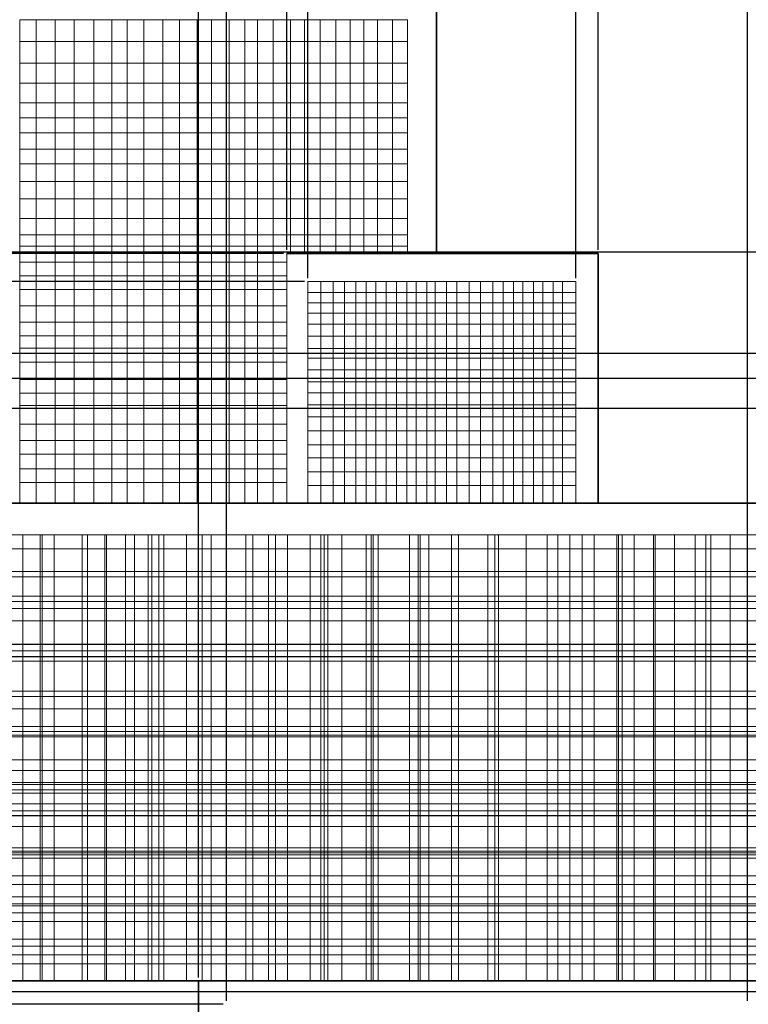
# Model space of a CAD drawing. Units: inches. Extents: x -10 to 130, y -32 to 34.
# Tile 9 of 22: x 28.66 to 42.14, y 5.57 to 23.78. Entities that reach past the tile are written whole.
import ezdxf

# ---------------------------------------------------------------- set-up
doc = ezdxf.new("R2010")
doc.units = ezdxf.units.IN
doc.header["$MEASUREMENT"] = 0
for name, color, linetype, lineweight in [('A-ANNO-DIMS', 2, 'Continuous', 18), ('A-ELEV', 7, 'Continuous', 35), ('A-GLAZ', 4, 'Continuous', 18)]:
    doc.layers.add(name, color=color, linetype=linetype, lineweight=lineweight)
doc.styles.get("Standard").update_dxf_attribs({"font": 'arial.ttf'})
doc.dimstyles.get("Standard").update_dxf_attribs({"dimtxt": 0.18, "dimasz": 0.18, "dimexe": 0.18, "dimexo": 0.0625, "dimgap": 0.09, "dimtad": 0, "dimtih": 1, "dimtoh": 1, "dimdec": 4, "dimzin": 0, "dimdsep": 46, "dimtxsty": 'Standard', "dimcen": 0.09, "dimadec": 0, "dimazin": 0, "dimtfac": 1, "dimtdec": 4, "dimtofl": 0, "dimtmove": 0, "dimatfit": 3, "dimfxl": 1, "dimtolj": 1, "dimtzin": 0, "dimarcsym": 0})

# ---------------------------------------------------------------- blocks, each defined once
blk = doc.blocks.new('*D5')
at = {"layer": 'A-ANNO-DIMS', "color": 0, "lineweight": -2, "transparency": 16777216}
for p, q in [((26.399, 6.07), (26.399, 33.879)), ((31.971, 6.07), (31.971, 33.879)), ((26.579, 33.699), (28.792, 33.699)), ((31.791, 33.699), (29.578, 33.699))]:
    blk.add_line(p, q, dxfattribs=at)
at = {"layer": 'A-ANNO-DIMS', "color": 0, "transparency": 16777216}
for points in [[(26.579, 33.729), (26.579, 33.669), (26.399, 33.699)], [(31.791, 33.729), (31.791, 33.669), (31.971, 33.699)]]:
    blk.add_solid(points, dxfattribs=at)
at = {"layer": 'Defpoints', "color": 0, "transparency": 16777216}
for p in [(31.971, 33.699), (26.399, 6.007), (31.971, 6.007)]:
    blk.add_point(p, dxfattribs=at)
at = {"layer": 'A-ANNO-DIMS', "color": 0, "transparency": 16777216, "insert": (29.185, 33.699), "char_height": 0.18, "attachment_point": 5}
blk.add_mtext('\\A1;5.572', dxfattribs=at)
blk = doc.blocks.new('*D6')
at = {"layer": 'A-ANNO-DIMS', "color": 0, "lineweight": -2, "transparency": 16777216}
for p, q in [((31.971, 6.07), (31.971, 33.879)), ((42.614, 6.07), (42.614, 33.879)), ((32.151, 33.699), (36.837, 33.699)), ((42.434, 33.699), (37.748, 33.699))]:
    blk.add_line(p, q, dxfattribs=at)
at = {"layer": 'A-ANNO-DIMS', "color": 0, "transparency": 16777216}
for points in [[(32.151, 33.729), (32.151, 33.669), (31.971, 33.699)], [(42.434, 33.729), (42.434, 33.669), (42.614, 33.699)]]:
    blk.add_solid(points, dxfattribs=at)
at = {"layer": 'Defpoints', "color": 0, "transparency": 16777216}
for p in [(42.614, 33.699), (31.971, 6.007), (42.614, 6.007)]:
    blk.add_point(p, dxfattribs=at)
at = {"layer": 'A-ANNO-DIMS', "color": 0, "transparency": 16777216, "insert": (37.293, 33.699), "char_height": 0.18, "attachment_point": 5}
blk.add_mtext('\\A1;10.643', dxfattribs=at)
blk = doc.blocks.new('*D14')
at = {"layer": 'A-ANNO-DIMS', "color": 0, "lineweight": -2, "transparency": 16777216}
for p, q in [((28.1, 24.464), (28.1, 33.879)), ((33.608, 19.52), (33.608, 33.879)), ((28.28, 33.699), (30.46, 33.699)), ((33.428, 33.699), (31.248, 33.699))]:
    blk.add_line(p, q, dxfattribs=at)
at = {"layer": 'A-ANNO-DIMS', "color": 0, "transparency": 16777216}
for points in [[(28.28, 33.729), (28.28, 33.669), (28.1, 33.699)], [(33.428, 33.729), (33.428, 33.669), (33.608, 33.699)]]:
    blk.add_solid(points, dxfattribs=at)
at = {"layer": 'Defpoints', "color": 0, "transparency": 16777216}
for p in [(33.608, 33.699), (28.1, 24.402), (33.608, 19.458)]:
    blk.add_point(p, dxfattribs=at)
at = {"layer": 'A-ANNO-DIMS', "color": 0, "transparency": 16777216, "insert": (30.854, 33.699), "char_height": 0.18, "attachment_point": 5}
blk.add_mtext('\\A1;5.508', dxfattribs=at)
blk = doc.blocks.new('*D15')
at = {"layer": 'A-ANNO-DIMS', "color": 0, "lineweight": -2, "transparency": 16777216}
for p, q in [((33.608, 19.52), (33.608, 33.879)), ((36.377, 24.464), (36.377, 33.879)), ((33.788, 33.699), (34.597, 33.699)), ((36.197, 33.699), (35.388, 33.699))]:
    blk.add_line(p, q, dxfattribs=at)
at = {"layer": 'A-ANNO-DIMS', "color": 0, "transparency": 16777216}
for points in [[(33.788, 33.729), (33.788, 33.669), (33.608, 33.699)], [(36.197, 33.729), (36.197, 33.669), (36.377, 33.699)]]:
    blk.add_solid(points, dxfattribs=at)
at = {"layer": 'Defpoints', "color": 0, "transparency": 16777216}
for p in [(36.377, 33.699), (36.377, 24.402), (33.608, 19.458)]:
    blk.add_point(p, dxfattribs=at)
at = {"layer": 'A-ANNO-DIMS', "color": 0, "transparency": 16777216, "insert": (34.993, 33.699), "char_height": 0.18, "attachment_point": 5}
blk.add_mtext('\\A1;2.769', dxfattribs=at)
blk = doc.blocks.new('*D16')
at = {"layer": 'A-ANNO-DIMS', "color": 0, "lineweight": -2, "transparency": 16777216}
for p, q in [((36.377, 24.464), (36.377, 33.879)), ((39.364, 19.52), (39.364, 33.879)), ((36.557, 33.699), (37.476, 33.699)), ((39.184, 33.699), (38.266, 33.699))]:
    blk.add_line(p, q, dxfattribs=at)
at = {"layer": 'A-ANNO-DIMS', "color": 0, "transparency": 16777216}
for points in [[(36.557, 33.729), (36.557, 33.669), (36.377, 33.699)], [(39.184, 33.729), (39.184, 33.669), (39.364, 33.699)]]:
    blk.add_solid(points, dxfattribs=at)
at = {"layer": 'Defpoints', "color": 0, "transparency": 16777216}
for p in [(39.364, 33.699), (36.377, 24.402), (39.364, 19.458)]:
    blk.add_point(p, dxfattribs=at)
at = {"layer": 'A-ANNO-DIMS', "color": 0, "transparency": 16777216, "insert": (37.871, 33.699), "char_height": 0.18, "attachment_point": 5}
blk.add_mtext('\\A1;2.987', dxfattribs=at)
blk = doc.blocks.new('*D17')
at = {"layer": 'A-ANNO-DIMS', "color": 0, "lineweight": -2, "transparency": 16777216}
for p, q in [((39.364, 19.52), (39.364, 33.879)), ((44.622, 17.67), (44.622, 33.879)), ((39.544, 33.699), (41.599, 33.699)), ((44.442, 33.699), (42.387, 33.699))]:
    blk.add_line(p, q, dxfattribs=at)
at = {"layer": 'A-ANNO-DIMS', "color": 0, "transparency": 16777216}
for points in [[(39.544, 33.729), (39.544, 33.669), (39.364, 33.699)], [(44.442, 33.729), (44.442, 33.669), (44.622, 33.699)]]:
    blk.add_solid(points, dxfattribs=at)
at = {"layer": 'Defpoints', "color": 0, "transparency": 16777216}
for p in [(44.622, 33.699), (39.364, 19.458), (44.622, 17.607)]:
    blk.add_point(p, dxfattribs=at)
at = {"layer": 'A-ANNO-DIMS', "color": 0, "transparency": 16777216, "insert": (41.993, 33.699), "char_height": 0.18, "attachment_point": 5}
blk.add_mtext('\\A1;5.257', dxfattribs=at)
blk = doc.blocks.new('*D28')
at = {"layer": 'A-ANNO-DIMS', "color": 0, "lineweight": -2, "transparency": 16777216}
for p, q in [((21.715, 14.903), (21.715, 33.879)), ((49.946, 14.903), (49.946, 33.879)), ((21.895, 33.699), (35.436, 33.699)), ((49.766, 33.699), (36.226, 33.699))]:
    blk.add_line(p, q, dxfattribs=at)
at = {"layer": 'A-ANNO-DIMS', "color": 0, "transparency": 16777216}
for points in [[(21.895, 33.729), (21.895, 33.669), (21.715, 33.699)], [(49.766, 33.729), (49.766, 33.669), (49.946, 33.699)]]:
    blk.add_solid(points, dxfattribs=at)
at = {"layer": 'Defpoints', "color": 0, "transparency": 16777216}
for p in [(49.946, 33.699), (21.715, 14.841), (49.946, 14.841)]:
    blk.add_point(p, dxfattribs=at)
at = {"layer": 'A-ANNO-DIMS', "color": 0, "transparency": 16777216, "insert": (35.831, 33.699), "char_height": 0.18, "attachment_point": 5}
blk.add_mtext('\\A1;28.23', dxfattribs=at)
blk = doc.blocks.new('*D34')
at = {"layer": 'A-ANNO-DIMS', "color": 0, "lineweight": -2, "transparency": 16777216}
for p, q in [((13.34, 6.007), (-9.564, 6.007)), ((-9.384, 5.827), (-9.384, 3.941)), ((-9.384, 1.691), (-9.384, 3.577)), ((70.835, 1.511), (-9.564, 1.511))]:
    blk.add_line(p, q, dxfattribs=at)
at = {"layer": 'A-ANNO-DIMS', "color": 0, "transparency": 16777216}
for points in [[(-9.414, 5.827), (-9.354, 5.827), (-9.384, 6.007)], [(-9.414, 1.691), (-9.354, 1.691), (-9.384, 1.511)]]:
    blk.add_solid(points, dxfattribs=at)
at = {"layer": 'Defpoints', "color": 0, "transparency": 16777216}
for p in [(-9.384, 6.007), (13.402, 6.007), (70.898, 1.511)]:
    blk.add_point(p, dxfattribs=at)
at = {"layer": 'A-ANNO-DIMS', "color": 0, "transparency": 16777216, "insert": (-9.384, 3.759), "char_height": 0.18, "attachment_point": 5}
blk.add_mtext('\\A1;4.497', dxfattribs=at)
blk = doc.blocks.new('*D36')
at = {"layer": 'A-ANNO-DIMS', "color": 0, "lineweight": -2, "transparency": 16777216}
for p, q in [((44.559, 17.607), (-9.564, 17.607)), ((-9.384, 17.427), (-9.384, 16.405)), ((-9.384, 15.021), (-9.384, 16.044)), ((21.653, 14.841), (-9.564, 14.841))]:
    blk.add_line(p, q, dxfattribs=at)
at = {"layer": 'A-ANNO-DIMS', "color": 0, "transparency": 16777216}
for points in [[(-9.414, 17.427), (-9.354, 17.427), (-9.384, 17.607)], [(-9.414, 15.021), (-9.354, 15.021), (-9.384, 14.841)]]:
    blk.add_solid(points, dxfattribs=at)
at = {"layer": 'Defpoints', "color": 0, "transparency": 16777216}
for p in [(-9.384, 17.607), (44.622, 17.607), (21.715, 14.841)]:
    blk.add_point(p, dxfattribs=at)
at = {"layer": 'A-ANNO-DIMS', "color": 0, "transparency": 16777216, "insert": (-9.384, 16.224), "char_height": 0.18, "attachment_point": 5}
blk.add_mtext('\\A1;2.77', dxfattribs=at)
blk = doc.blocks.new('*D37')
at = {"layer": 'A-ANNO-DIMS', "color": 0, "lineweight": -2, "transparency": 16777216}
for p, q in [((19.526, 19.485), (-9.564, 19.485)), ((-9.384, 19.305), (-9.384, 18.728)), ((-9.384, 17.787), (-9.384, 18.364)), ((44.559, 17.607), (-9.564, 17.607))]:
    blk.add_line(p, q, dxfattribs=at)
at = {"layer": 'A-ANNO-DIMS', "color": 0, "transparency": 16777216}
for points in [[(-9.414, 19.305), (-9.354, 19.305), (-9.384, 19.485)], [(-9.414, 17.787), (-9.354, 17.787), (-9.384, 17.607)]]:
    blk.add_solid(points, dxfattribs=at)
at = {"layer": 'Defpoints', "color": 0, "transparency": 16777216}
for p in [(-9.384, 19.485), (19.588, 19.485), (44.622, 17.607)]:
    blk.add_point(p, dxfattribs=at)
at = {"layer": 'A-ANNO-DIMS', "color": 0, "transparency": 16777216, "insert": (-9.384, 18.546), "char_height": 0.18, "attachment_point": 5}
blk.add_mtext('\\A1;1.877', dxfattribs=at)
blk = doc.blocks.new('*D74')
at = {"layer": 'A-ANNO-DIMS', "color": 0, "lineweight": -2, "transparency": 16777216}
for p, q in [((54.085, 17.607), (-9.564, 17.607)), ((-9.384, 17.427), (-9.384, 17.281)), ((-9.384, 16.771), (-9.384, 16.917)), ((55.856, 16.591), (-9.564, 16.591))]:
    blk.add_line(p, q, dxfattribs=at)
at = {"layer": 'A-ANNO-DIMS', "color": 0, "transparency": 16777216}
for points in [[(-9.414, 17.427), (-9.354, 17.427), (-9.384, 17.607)], [(-9.414, 16.771), (-9.354, 16.771), (-9.384, 16.591)]]:
    blk.add_solid(points, dxfattribs=at)
at = {"layer": 'Defpoints', "color": 0, "transparency": 16777216}
for p in [(54.147, 17.607), (-9.384, 16.591), (55.918, 16.591)]:
    blk.add_point(p, dxfattribs=at)
at = {"layer": 'A-ANNO-DIMS', "color": 0, "transparency": 16777216, "insert": (-9.384, 17.099), "char_height": 0.18, "attachment_point": 5}
blk.add_mtext('\\A1;1.02', dxfattribs=at)
blk = doc.blocks.new('*D82')
at = {"layer": 'A-ANNO-DIMS', "color": 0, "lineweight": -2, "transparency": 16777216}
for p, q in [((19.651, 19.485), (129.508, 19.485)), ((129.328, 19.305), (129.328, 18.728)), ((129.328, 17.787), (129.328, 18.364)), ((68.738, 17.607), (129.508, 17.607))]:
    blk.add_line(p, q, dxfattribs=at)
at = {"layer": 'A-ANNO-DIMS', "color": 0, "transparency": 16777216}
for points in [[(129.298, 19.305), (129.358, 19.305), (129.328, 19.485)], [(129.298, 17.787), (129.358, 17.787), (129.328, 17.607)]]:
    blk.add_solid(points, dxfattribs=at)
at = {"layer": 'Defpoints', "color": 0, "transparency": 16777216}
for p in [(19.588, 19.485), (68.676, 17.607), (129.328, 17.607)]:
    blk.add_point(p, dxfattribs=at)
at = {"layer": 'A-ANNO-DIMS', "color": 0, "transparency": 16777216, "insert": (129.328, 18.546), "char_height": 0.18, "attachment_point": 5}
blk.add_mtext('\\A1;1.877', dxfattribs=at)
blk = doc.blocks.new('*D87')
at = {"layer": 'A-ANNO-DIMS', "color": 0, "lineweight": -2, "transparency": 16777216}
for p, q in [((49.884, 14.841), (-9.564, 14.841)), ((-9.384, 14.661), (-9.384, 13.713)), ((-9.384, 12.402), (-9.384, 13.35)), ((49.884, 12.222), (-9.564, 12.222))]:
    blk.add_line(p, q, dxfattribs=at)
at = {"layer": 'A-ANNO-DIMS', "color": 0, "transparency": 16777216}
for points in [[(-9.414, 14.661), (-9.354, 14.661), (-9.384, 14.841)], [(-9.414, 12.402), (-9.354, 12.402), (-9.384, 12.222)]]:
    blk.add_solid(points, dxfattribs=at)
at = {"layer": 'Defpoints', "color": 0, "transparency": 16777216}
for p in [(49.946, 14.841), (-9.384, 12.222), (49.946, 12.222)]:
    blk.add_point(p, dxfattribs=at)
at = {"layer": 'A-ANNO-DIMS', "color": 0, "transparency": 16777216, "insert": (-9.384, 13.532), "char_height": 0.18, "attachment_point": 5}
blk.add_mtext('\\A1;2.619', dxfattribs=at)
blk = doc.blocks.new('*D88')
at = {"layer": 'A-ANNO-DIMS', "color": 0, "lineweight": -2, "transparency": 16777216}
for p, q in [((49.884, 12.222), (-9.564, 12.222)), ((-9.384, 12.042), (-9.384, 10.822)), ((-9.384, 9.238), (-9.384, 10.458)), ((49.884, 9.058), (-9.564, 9.058))]:
    blk.add_line(p, q, dxfattribs=at)
at = {"layer": 'A-ANNO-DIMS', "color": 0, "transparency": 16777216}
for points in [[(-9.414, 12.042), (-9.354, 12.042), (-9.384, 12.222)], [(-9.414, 9.238), (-9.354, 9.238), (-9.384, 9.058)]]:
    blk.add_solid(points, dxfattribs=at)
at = {"layer": 'Defpoints', "color": 0, "transparency": 16777216}
for p in [(49.946, 12.222), (-9.384, 9.058), (49.946, 9.058)]:
    blk.add_point(p, dxfattribs=at)
at = {"layer": 'A-ANNO-DIMS', "color": 0, "transparency": 16777216, "insert": (-9.384, 10.64), "char_height": 0.18, "attachment_point": 5}
blk.add_mtext('\\A1;3.164', dxfattribs=at)
blk = doc.blocks.new('*D89')
at = {"layer": 'A-ANNO-DIMS', "color": 0, "lineweight": -2, "transparency": 16777216}
for p, q in [((49.884, 9.058), (-9.564, 9.058)), ((-9.384, 8.878), (-9.384, 7.612)), ((-9.384, 5.982), (-9.384, 7.248)), ((49.884, 5.802), (-9.564, 5.802))]:
    blk.add_line(p, q, dxfattribs=at)
at = {"layer": 'A-ANNO-DIMS', "color": 0, "transparency": 16777216}
for points in [[(-9.414, 8.878), (-9.354, 8.878), (-9.384, 9.058)], [(-9.414, 5.982), (-9.354, 5.982), (-9.384, 5.802)]]:
    blk.add_solid(points, dxfattribs=at)
at = {"layer": 'Defpoints', "color": 0, "transparency": 16777216}
for p in [(49.946, 9.058), (-9.384, 5.802), (49.946, 5.802)]:
    blk.add_point(p, dxfattribs=at)
at = {"layer": 'A-ANNO-DIMS', "color": 0, "transparency": 16777216, "insert": (-9.384, 7.43), "char_height": 0.18, "attachment_point": 5}
blk.add_mtext('\\A1;3.256', dxfattribs=at)
blk = doc.blocks.new('*D90')
at = {"layer": 'A-ANNO-DIMS', "color": 0, "lineweight": -2, "transparency": 16777216}
for p, q in [((49.884, 5.802), (-9.564, 5.802)), ((-9.384, 5.622), (-9.384, 4.421)), ((-9.384, 2.855), (-9.384, 4.057)), ((49.884, 2.675), (-9.564, 2.675))]:
    blk.add_line(p, q, dxfattribs=at)
at = {"layer": 'A-ANNO-DIMS', "color": 0, "transparency": 16777216}
for points in [[(-9.414, 5.622), (-9.354, 5.622), (-9.384, 5.802)], [(-9.414, 2.855), (-9.354, 2.855), (-9.384, 2.675)]]:
    blk.add_solid(points, dxfattribs=at)
at = {"layer": 'Defpoints', "color": 0, "transparency": 16777216}
for p in [(49.946, 5.802), (-9.384, 2.675), (49.946, 2.675)]:
    blk.add_point(p, dxfattribs=at)
at = {"layer": 'A-ANNO-DIMS', "color": 0, "transparency": 16777216, "insert": (-9.384, 4.239), "char_height": 0.18, "attachment_point": 5}
blk.add_mtext('\\A1;3.127', dxfattribs=at)
blk = doc.blocks.new('*D95')
at = {"layer": 'A-ANNO-DIMS', "color": 0, "lineweight": -2, "transparency": 16777216}
for p, q in [((-9.384, 12.402), (-9.384, 12.582)), ((49.884, 12.222), (-9.564, 12.222)), ((49.884, 11.995), (-9.564, 11.995)), ((-9.384, 11.815), (-9.384, 11.635)), ((-9.384, 11.635), (-9.564, 11.635))]:
    blk.add_line(p, q, dxfattribs=at)
at = {"layer": 'A-ANNO-DIMS', "color": 0, "transparency": 16777216}
for points in [[(-9.414, 12.402), (-9.354, 12.402), (-9.384, 12.222)], [(-9.414, 11.815), (-9.354, 11.815), (-9.384, 11.995)]]:
    blk.add_solid(points, dxfattribs=at)
at = {"layer": 'Defpoints', "color": 0, "transparency": 16777216}
for p in [(49.946, 12.222), (-9.384, 11.995), (49.946, 11.995)]:
    blk.add_point(p, dxfattribs=at)
at = {"layer": 'A-ANNO-DIMS', "color": 0, "transparency": 16777216, "insert": (-9.957, 11.635), "char_height": 0.18, "attachment_point": 5}
blk.add_mtext('\\A1;0.227', dxfattribs=at)
blk = doc.blocks.new('*D102')
at = {"layer": 'A-ANNO-DIMS', "color": 0, "lineweight": -2, "transparency": 16777216}
for p, q in [((33.608, 19.52), (33.608, 33.879)), ((33.994, 18.998), (33.994, 33.879)), ((33.428, 33.699), (33.248, 33.699)), ((34.174, 33.699), (34.354, 33.699))]:
    blk.add_line(p, q, dxfattribs=at)
at = {"layer": 'A-ANNO-DIMS', "color": 0, "transparency": 16777216}
for points in [[(33.428, 33.729), (33.428, 33.669), (33.608, 33.699)], [(34.174, 33.729), (34.174, 33.669), (33.994, 33.699)]]:
    blk.add_solid(points, dxfattribs=at)
at = {"layer": 'Defpoints', "color": 0, "transparency": 16777216}
for p in [(33.994, 33.699), (33.608, 19.458), (33.994, 18.936)]:
    blk.add_point(p, dxfattribs=at)
at = {"layer": 'A-ANNO-DIMS', "color": 0, "transparency": 16777216, "insert": (34.748, 33.699), "char_height": 0.18, "attachment_point": 5}
blk.add_mtext('\\A1;0.386', dxfattribs=at)
blk = doc.blocks.new('*D103')
at = {"layer": 'A-ANNO-DIMS', "color": 0, "lineweight": -2, "transparency": 16777216}
for p, q in [((33.994, 18.998), (33.994, 33.879)), ((38.954, 18.998), (38.954, 33.879)), ((34.174, 33.699), (36.077, 33.699)), ((38.774, 33.699), (36.871, 33.699))]:
    blk.add_line(p, q, dxfattribs=at)
at = {"layer": 'A-ANNO-DIMS', "color": 0, "transparency": 16777216}
for points in [[(34.174, 33.729), (34.174, 33.669), (33.994, 33.699)], [(38.774, 33.729), (38.774, 33.669), (38.954, 33.699)]]:
    blk.add_solid(points, dxfattribs=at)
at = {"layer": 'Defpoints', "color": 0, "transparency": 16777216}
for p in [(38.954, 33.699), (33.994, 18.936), (38.954, 18.936)]:
    blk.add_point(p, dxfattribs=at)
at = {"layer": 'A-ANNO-DIMS', "color": 0, "transparency": 16777216, "insert": (36.474, 33.699), "char_height": 0.18, "attachment_point": 5}
blk.add_mtext('\\A1;4.960', dxfattribs=at)
blk = doc.blocks.new('*D104')
at = {"layer": 'A-ANNO-DIMS', "color": 0, "lineweight": -2, "transparency": 16777216}
for p, q in [((-9.383551, 19.637521), (-9.383551, 19.817521)), ((33.54566, 19.457521), (-9.563551, 19.457521)), ((33.931459, 18.935883), (-9.563551, 18.935883)), ((-9.383551, 18.755883), (-9.383551, 18.575883))]:
    blk.add_line(p, q, dxfattribs=at)
at = {"layer": 'A-ANNO-DIMS', "color": 0, "transparency": 16777216}
for points in [[(-9.413551, 19.637521), (-9.353551, 19.637521), (-9.383551, 19.457521)], [(-9.413551, 18.755883), (-9.353551, 18.755883), (-9.383551, 18.935883)]]:
    blk.add_solid(points, dxfattribs=at)
at = {"layer": 'Defpoints', "color": 0, "transparency": 16777216}
for p in [(-9.383551, 19.457521), (33.60816, 19.457521), (33.993959, 18.935883)]:
    blk.add_point(p, dxfattribs=at)
at = {"layer": 'A-ANNO-DIMS', "color": 0, "transparency": 16777216, "insert": (-9.383551, 19.196702), "char_height": 0.18, "attachment_point": 5}
blk.add_mtext('\\A1;0.522', dxfattribs=at)
blk = doc.blocks.new('*D106')
at = {"layer": 'A-ANNO-DIMS', "color": 0, "lineweight": -2, "transparency": 16777216}
for p, q in [((22.665, 14.318), (22.665, 33.879)), ((48.963, 14.318), (48.963, 33.879)), ((22.845, 33.699), (35.349, 33.699)), ((48.783, 33.699), (36.279, 33.699))]:
    blk.add_line(p, q, dxfattribs=at)
at = {"layer": 'A-ANNO-DIMS', "color": 0, "transparency": 16777216}
for points in [[(22.845, 33.729), (22.845, 33.669), (22.665, 33.699)], [(48.783, 33.729), (48.783, 33.669), (48.963, 33.699)]]:
    blk.add_solid(points, dxfattribs=at)
at = {"layer": 'Defpoints', "color": 0, "transparency": 16777216}
for p in [(48.963, 33.699), (22.665, 14.256), (48.963, 14.256)]:
    blk.add_point(p, dxfattribs=at)
at = {"layer": 'A-ANNO-DIMS', "color": 0, "transparency": 16777216, "insert": (35.814, 33.699), "char_height": 0.18, "attachment_point": 5}
blk.add_mtext('\\A1;26.298', dxfattribs=at)
blk = doc.blocks.new('*D110')
at = {"layer": 'A-ANNO-DIMS', "color": 0, "lineweight": -2, "transparency": 16777216}
for p, q in [((-9.383551, 17.787359), (-9.383551, 17.967359)), ((44.559228, 17.607359), (-9.563551, 17.607359)), ((45.040057, 17.142679), (-9.563551, 17.142679)), ((-9.383551, 16.962679), (-9.383551, 16.782679))]:
    blk.add_line(p, q, dxfattribs=at)
at = {"layer": 'A-ANNO-DIMS', "color": 0, "transparency": 16777216}
for points in [[(-9.413551, 17.787359), (-9.353551, 17.787359), (-9.383551, 17.607359)], [(-9.413551, 16.962679), (-9.353551, 16.962679), (-9.383551, 17.142679)]]:
    blk.add_solid(points, dxfattribs=at)
at = {"layer": 'Defpoints', "color": 0, "transparency": 16777216}
for p in [(-9.383551, 17.607359), (44.621728, 17.607359), (45.102557, 17.142679)]:
    blk.add_point(p, dxfattribs=at)
at = {"layer": 'A-ANNO-DIMS', "color": 0, "transparency": 16777216, "insert": (-9.383551, 17.375019), "char_height": 0.18, "attachment_point": 5}
blk.add_mtext('\\A1;0.465', dxfattribs=at)
blk = doc.blocks.new('*D119')
at = {"layer": 'A-ANNO-DIMS', "color": 0, "lineweight": -2, "transparency": 16777216}
for p, q in [((31.971, 6.07), (31.971, 33.879)), ((32.49, 5.634), (32.49, 33.879)), ((31.791, 33.699), (31.611, 33.699)), ((32.67, 33.699), (32.85, 33.699))]:
    blk.add_line(p, q, dxfattribs=at)
at = {"layer": 'A-ANNO-DIMS', "color": 0, "transparency": 16777216}
for points in [[(31.791, 33.729), (31.791, 33.669), (31.971, 33.699)], [(32.67, 33.729), (32.67, 33.669), (32.49, 33.699)]]:
    blk.add_solid(points, dxfattribs=at)
at = {"layer": 'Defpoints', "color": 0, "transparency": 16777216}
for p in [(32.49, 33.699), (31.971, 6.007), (32.49, 5.572)]:
    blk.add_point(p, dxfattribs=at)
at = {"layer": 'A-ANNO-DIMS', "color": 0, "transparency": 16777216, "insert": (33.244, 33.699), "char_height": 0.18, "attachment_point": 5}
blk.add_mtext('\\A1;0.519', dxfattribs=at)
blk = doc.blocks.new('*D120')
at = {"layer": 'A-ANNO-DIMS', "color": 0, "lineweight": -2, "transparency": 16777216}
for p, q in [((32.49, 5.634), (32.49, 33.879)), ((42.127, 5.634), (42.127, 33.879)), ((32.67, 33.699), (36.915, 33.699)), ((41.947, 33.699), (37.702, 33.699))]:
    blk.add_line(p, q, dxfattribs=at)
at = {"layer": 'A-ANNO-DIMS', "color": 0, "transparency": 16777216}
for points in [[(32.67, 33.729), (32.67, 33.669), (32.49, 33.699)], [(41.947, 33.729), (41.947, 33.669), (42.127, 33.699)]]:
    blk.add_solid(points, dxfattribs=at)
at = {"layer": 'Defpoints', "color": 0, "transparency": 16777216}
for p in [(42.127, 33.699), (32.49, 5.572), (42.127, 5.572)]:
    blk.add_point(p, dxfattribs=at)
at = {"layer": 'A-ANNO-DIMS', "color": 0, "transparency": 16777216, "insert": (37.308, 33.699), "char_height": 0.18, "attachment_point": 5}
blk.add_mtext('\\A1;9.637', dxfattribs=at)
blk = doc.blocks.new('*D121')
at = {"layer": 'A-ANNO-DIMS', "color": 0, "lineweight": -2, "transparency": 16777216}
for p, q in [((-9.384, 6.187), (-9.384, 6.367)), ((31.909, 6.007), (-9.564, 6.007)), ((32.427, 5.572), (-9.564, 5.572)), ((-9.384, 5.392), (-9.384, 5.212))]:
    blk.add_line(p, q, dxfattribs=at)
at = {"layer": 'A-ANNO-DIMS', "color": 0, "transparency": 16777216}
for points in [[(-9.414, 6.187), (-9.354, 6.187), (-9.384, 6.007)], [(-9.414, 5.392), (-9.354, 5.392), (-9.384, 5.572)]]:
    blk.add_solid(points, dxfattribs=at)
at = {"layer": 'Defpoints', "color": 0, "transparency": 16777216}
for p in [(-9.384, 6.007), (31.971, 6.007), (32.49, 5.572)]:
    blk.add_point(p, dxfattribs=at)
at = {"layer": 'A-ANNO-DIMS', "color": 0, "transparency": 16777216, "insert": (-9.384, 5.789), "char_height": 0.18, "attachment_point": 5}
blk.add_mtext('\\A1;0.436', dxfattribs=at)

msp = doc.modelspace()

# ---------------------------------------------------------------- linework, layer by layer
at = {"layer": 'A-ELEV'}
for p, q in [((36.3774, 24.4019), (36.3774, 19.4575)), ((36.3774, 19.4575), (33.6082, 19.4575)), ((36.3774, 19.4575), (39.3644, 19.4575)), ((39.3644, 19.4575), (39.3644, 14.8409)), ((21.7155, 14.8409), (49.9462, 14.8409)), ((20.3124, 6.0074), (49.9462, 6.0074)), ((31.9712, -6.2218), (31.9712, 6.0074))]:
    msp.add_line(p, q, dxfattribs=at)
at = {"layer": 'A-GLAZ'}
for p, q in [((28.6645, 23.7785), (28.6645, 14.8409)), ((28.6645, 23.7785), (35.841, 23.7785)), ((28.9723, 23.7785), (28.9723, 14.8409)), ((29.321, 23.7785), (29.321, 14.8409)), ((29.6697, 23.7785), (29.6697, 14.8409)), ((30.039, 23.7785), (30.039, 14.8409)), ((30.3672, 23.7785), (30.3672, 14.8409)), ((30.6545, 23.7785), (30.6545, 14.8409)), ((30.9622, 23.7785), (30.9622, 14.8409)), ((31.3109, 23.7785), (31.3109, 14.8409)), ((31.6186, 23.7785), (31.6186, 14.8409)), ((31.9469, 23.7785), (31.9469, 14.8409)), ((32.2136, 23.7785), (32.2136, 14.8409)), ((32.5418, 23.7785), (32.5418, 14.8409)), ((32.829, 23.7785), (32.829, 14.8409)), ((33.0672, 23.7785), (33.0672, 14.8409)), ((33.3515, 23.7785), (33.3515, 14.8409)), ((33.6779, 23.7785), (33.6779, 19.4575)), ((33.9309, 23.7785), (33.9309, 19.4575)), ((34.2218, 23.7785), (34.2218, 19.4575)), ((34.5128, 23.7785), (34.5128, 19.4575)), ((34.7784, 23.7785), (34.7784, 19.4575)), ((35.0314, 23.7785), (35.0314, 19.4575)), ((35.2844, 23.7785), (35.2844, 19.4575)), ((35.5627, 23.7785), (35.5627, 19.4575)), ((35.841, 23.7785), (35.841, 19.4575)), ((28.6645, 23.3752), (35.841, 23.3752)), ((28.6645, 22.9718), (35.841, 22.9718)), ((28.6645, 22.6051), (35.841, 22.6051)), ((28.6645, 22.2381), (35.841, 22.2381)), ((28.6645, 21.9622), (35.841, 21.9622)), ((28.6645, 21.6862), (35.841, 21.6862)), ((28.6645, 21.3872), (35.841, 21.3872)), ((28.6645, 21.1112), (35.841, 21.1112)), ((28.6645, 20.7893), (35.841, 20.7893)), ((28.6645, 20.4673), (35.841, 20.4673)), ((28.6645, 20.0993), (35.841, 20.0993)), ((28.6645, 19.8003), (35.841, 19.8003)), ((28.6645, 19.5933), (35.841, 19.5933)), ((33.6082, 19.4575), (33.6082, 14.8409)), ((28.6645, 19.2944), (33.6082, 19.2944)), ((28.6645, 19.0414), (33.6082, 19.0414)), ((36.3774, 18.9359), (33.994, 18.9359)), ((33.994, 18.9359), (33.994, 14.8409)), ((34.2385, 18.9359), (34.2385, 14.8409)), ((34.4656, 18.9359), (34.4656, 14.8409)), ((34.6752, 18.9359), (34.6752, 14.8409)), ((34.8848, 18.9359), (34.8848, 14.8409)), ((35.0769, 18.9359), (35.0769, 14.8409)), ((35.2515, 18.9359), (35.2515, 14.8409)), ((35.4437, 18.9359), (35.4437, 14.8409)), ((35.6358, 18.9359), (35.6358, 14.8409)), ((35.8279, 18.9359), (35.8279, 14.8409)), ((36.0026, 18.9359), (36.0026, 14.8409)), ((36.1947, 18.9359), (36.1947, 14.8409)), ((36.3519, 18.9359), (36.3519, 14.8409)), ((36.3774, 18.9359), (38.9544, 18.9359)), ((36.5615, 18.9359), (36.5615, 14.8409)), ((36.7537, 18.9359), (36.7537, 14.8409)), ((36.9807, 18.9359), (36.9807, 14.8409)), ((37.1903, 18.9359), (37.1903, 14.8409)), ((37.4171, 18.9359), (37.4171, 14.8409)), ((37.6092, 18.9359), (37.6092, 14.8409)), ((37.8013, 18.9359), (37.8013, 14.8409)), ((37.976, 18.9359), (37.976, 14.8409)), ((38.1681, 18.9359), (38.1681, 14.8409)), ((38.3428, 18.9359), (38.3428, 14.8409)), ((38.5349, 18.9359), (38.5349, 14.8409)), ((38.7096, 18.9359), (38.7096, 14.8409)), ((38.9544, 18.9359), (38.9544, 14.8409)), ((28.6645, 18.7884), (33.6082, 18.7884)), ((36.3774, 18.7336), (33.994, 18.7336)), ((36.3774, 18.7336), (38.9544, 18.7336)), ((28.6645, 18.4894), (33.6082, 18.4894)), ((36.3774, 18.5419), (33.994, 18.5419)), ((36.3774, 18.5419), (38.9544, 18.5419)), ((36.3774, 18.3502), (33.994, 18.3502)), ((36.3774, 18.3502), (38.9544, 18.3502)), ((28.6645, 18.1847), (33.6082, 18.1847)), ((36.3774, 18.1479), (33.994, 18.1479)), ((36.3774, 18.1479), (38.9544, 18.1479)), ((28.6645, 17.9317), (33.6082, 17.9317)), ((36.3774, 17.9243), (33.994, 17.9243)), ((36.3774, 17.9243), (38.9544, 17.9243)), ((28.6645, 17.7017), (33.6082, 17.7017)), ((36.3774, 17.7007), (33.994, 17.7007)), ((36.3774, 17.7007), (38.9544, 17.7007)), ((36.3774, 17.5197), (33.994, 17.5197)), ((36.3774, 17.5197), (38.9544, 17.5197)), ((28.6645, 17.4487), (33.6082, 17.4487)), ((36.3774, 17.3067), (33.994, 17.3067)), ((36.3774, 17.3067), (38.9544, 17.3067)), ((28.6645, 17.1267), (33.6082, 17.1267)), ((36.3774, 17.0831), (33.994, 17.0831)), ((36.3774, 17.0831), (38.9544, 17.0831)), ((28.6645, 16.8738), (33.6082, 16.8738)), ((36.3774, 16.8808), (33.994, 16.8808)), ((36.3774, 16.8808), (38.9544, 16.8808)), ((28.6645, 16.6438), (33.6082, 16.6438)), ((36.3774, 16.6571), (33.994, 16.6571)), ((36.3774, 16.6571), (38.9544, 16.6571)), ((36.3774, 16.4335), (33.994, 16.4335)), ((36.3774, 16.4335), (38.9544, 16.4335)), ((28.6645, 16.2988), (33.6082, 16.2988)), ((36.3774, 16.1747), (33.994, 16.1747)), ((36.3774, 16.1747), (38.9544, 16.1747)), ((28.6645, 15.9998), (33.6082, 15.9998)), ((36.3774, 15.9192), (33.994, 15.9192)), ((36.3774, 15.9192), (38.9544, 15.9192)), ((28.6645, 15.7469), (33.6082, 15.7469)), ((36.3774, 15.6742), (33.994, 15.6742)), ((36.3774, 15.6742), (38.9544, 15.6742)), ((28.6645, 15.4709), (33.6082, 15.4709)), ((36.3774, 15.4187), (33.994, 15.4187)), ((36.3774, 15.4187), (38.9544, 15.4187)), ((28.6645, 15.2179), (33.6082, 15.2179)), ((36.3774, 15.1631), (33.994, 15.1631)), ((36.3774, 15.1631), (38.9544, 15.1631)), ((22.6649, 14.2556), (48.963, 14.2556)), ((28.7237, 6.0074), (28.7237, 14.2556)), ((28.7237, 6.0074), (28.7237, 14.2556)), ((29.046, 6.0074), (29.046, 14.2556)), ((29.0782, 6.0074), (29.0782, 14.2556)), ((29.3038, 6.0074), (29.3038, 14.2556)), ((29.8195, 6.0074), (29.8195, 14.2556)), ((29.9162, 6.0074), (29.9162, 14.2556)), ((30.2385, 6.0074), (30.2385, 14.2556)), ((30.2707, 6.0074), (30.2707, 14.2556)), ((30.6252, 6.0074), (30.6252, 14.2556)), ((30.7863, 6.0074), (30.7863, 14.2556)), ((30.7863, 6.0074), (30.7863, 14.2556)), ((31.0442, 6.0074), (31.0442, 14.2556)), ((31.1086, 6.0074), (31.1086, 14.2556)), ((31.2375, 6.0074), (31.2375, 14.2556)), ((31.3342, 6.0074), (31.3342, 14.2556)), ((31.7532, 6.0074), (31.7532, 14.2556)), ((32.0432, 6.0074), (32.0432, 14.2556)), ((32.2044, 6.0074), (32.2044, 14.2556)), ((32.8489, 6.0074), (32.8489, 14.2556)), ((32.9778, 6.0074), (32.9778, 14.2556)), ((33.2679, 6.0074), (33.2679, 14.2556)), ((33.2679, 6.0074), (33.2679, 14.2556)), ((33.3968, 6.0074), (33.3968, 14.2556)), ((33.6224, 6.0074), (33.6224, 14.2556)), ((34.0414, 6.0074), (34.0414, 14.2556)), ((34.2347, 6.0074), (34.2347, 14.2556)), ((34.2992, 6.0074), (34.2992, 14.2556)), ((34.3637, 6.0074), (34.3637, 14.2556)), ((34.6215, 6.0074), (34.6215, 14.2556)), ((35.0727, 6.0074), (35.0727, 14.2556)), ((35.1694, 6.0074), (35.1694, 14.2556)), ((35.2016, 6.0074), (35.2016, 14.2556)), ((35.2983, 6.0074), (35.2983, 14.2556)), ((35.8784, 6.0074), (35.8784, 14.2556)), ((36.0395, 6.0074), (36.0395, 14.2556)), ((36.0717, 6.0074), (36.0717, 14.2556)), ((36.2329, 6.0074), (36.2329, 14.2556)), ((36.6519, 6.0074), (36.6519, 14.2556)), ((36.6519, 6.0074), (36.6519, 14.2556)), ((36.7808, 6.0074), (36.7808, 14.2556)), ((37.3286, 6.0074), (37.3286, 14.2556)), ((37.3286, 6.0074), (37.3286, 14.2556)), ((37.4576, 6.0074), (37.4576, 14.2556)), ((37.522, 6.0074), (37.522, 14.2556)), ((38.0377, 6.0074), (38.0377, 14.2556)), ((38.4244, 6.0074), (38.4244, 14.2556)), ((38.4244, 6.0074), (38.4244, 14.2556)), ((38.6178, 6.0074), (38.6178, 14.2556)), ((38.8434, 6.0074), (38.8434, 14.2556)), ((39.069, 6.0074), (39.069, 14.2556)), ((39.2946, 6.0074), (39.2946, 14.2556)), ((39.7135, 6.0074), (39.7135, 14.2556)), ((39.7457, 6.0074), (39.7457, 14.2556)), ((39.8102, 6.0074), (39.8102, 14.2556)), ((40.0358, 6.0074), (40.0358, 14.2556)), ((40.3903, 6.0074), (40.3903, 14.2556)), ((40.4225, 6.0074), (40.4225, 14.2556)), ((40.777, 6.0074), (40.777, 14.2556)), ((41.1638, 6.0074), (41.1638, 14.2556)), ((41.3572, 6.0074), (41.3572, 14.2556)), ((41.4538, 6.0074), (41.4538, 14.2556)), ((41.8083, 6.0074), (41.8083, 14.2556)), ((22.6649, 13.9954), (48.963, 13.9954)), ((22.6649, 13.5727), (48.963, 13.5727)), ((22.6649, 13.4751), (48.963, 13.4751)), ((22.6649, 13.1174), (48.963, 13.1174)), ((22.6649, 13.0199), (48.963, 13.0199)), ((22.6649, 12.8898), (48.963, 12.8898)), ((22.6649, 12.8898), (48.963, 12.8898)), ((22.6649, 12.6622), (48.963, 12.6622)), ((22.6649, 12.1093), (48.963, 12.1093)), ((22.6649, 11.9142), (48.963, 11.9142)), ((22.6649, 11.3614), (48.963, 11.3614)), ((22.6649, 11.3614), (48.963, 11.3614)), ((22.6649, 11.2638), (48.963, 11.2638)), ((22.6649, 11.0362), (48.963, 11.0362)), ((22.6649, 10.711), (48.963, 10.711)), ((22.6649, 10.711), (48.963, 10.711)), ((22.6649, 10.711), (48.963, 10.711)), ((22.6649, 10.6134), (48.963, 10.6134)), ((22.6649, 10.5484), (48.963, 10.5484)), ((22.6649, 10.5159), (48.963, 10.5159)), ((22.6649, 10.0931), (48.963, 10.0931)), ((22.6649, 9.898), (48.963, 9.898)), ((22.6649, 9.6704), (48.963, 9.6704)), ((22.6649, 9.6379), (48.963, 9.6379)), ((22.6649, 9.5403), (48.963, 9.5403)), ((22.6649, 9.4753), (48.963, 9.4753)), ((22.6649, 9.2802), (48.963, 9.2802)), ((22.6649, 9.1501), (48.963, 9.1501)), ((22.6649, 8.8574), (48.963, 8.8574)), ((22.6649, 8.4672), (48.963, 8.4672)), ((22.6649, 8.4021), (48.963, 8.4021)), ((22.6649, 8.3696), (48.963, 8.3696)), ((22.6649, 8.3371), (48.963, 8.3371)), ((22.6649, 8.2721), (48.963, 8.2721)), ((22.6649, 7.9469), (48.963, 7.9469)), ((22.6649, 7.7843), (48.963, 7.7843)), ((22.6649, 7.5566), (48.963, 7.5566)), ((22.6649, 7.4266), (48.963, 7.4266)), ((22.6649, 7.3941), (48.963, 7.3941)), ((22.6649, 7.264), (48.963, 7.264)), ((22.6649, 7.1014), (48.963, 7.1014)), ((22.6649, 6.7762), (48.963, 6.7762)), ((22.6649, 6.6461), (48.963, 6.6461)), ((22.6649, 6.4835), (48.963, 6.4835)), ((22.6649, 6.3209), (48.963, 6.3209))]:
    msp.add_line(p, q, dxfattribs=at)

# ---------------------------------------------------------------- dimensions: what is measured, and where the dimension line sits
at = {"layer": 'A-ANNO-DIMS'}
for base, p1, p2, override, picture, middle in [((49.9462, 33.6987), (21.7155, 14.8409), (49.9462, 14.8409), {"dimdec": 2, "dimlfac": 1, "dimrnd": 0, "dimzin": 0, "dimdsep": 46, "dimlunit": 2}, '*D28', (35.8308, 33.6987)), ((48.963, 33.6987), (22.6649, 14.2556), (48.963, 14.2556), {"dimdec": 3, "dimlfac": 1, "dimrnd": 0, "dimzin": 0, "dimdsep": 46, "dimlunit": 2}, '*D106', (35.8139, 33.6987)), ((31.9712, 33.6987), (26.3988, 6.0074), (31.9712, 6.0074), {"dimdec": 3, "dimlfac": 1, "dimrnd": 0, "dimzin": 0, "dimdsep": 46, "dimlunit": 2}, '*D5', (29.185, 33.6987)), ((33.60816, 33.69866), (28.0997, 24.40191), (33.60816, 19.45752), {"dimdec": 3, "dimlfac": 1, "dimrnd": 0, "dimzin": 0, "dimdsep": 46, "dimlunit": 2}, '*D14', (30.85393, 33.69866)), ((32.4898, 33.6987), (31.9712, 6.0074), (32.4898, 5.5715), {"dimdec": 3, "dimlfac": 1, "dimrnd": 0, "dimzin": 0, "dimdsep": 46, "dimlunit": 2}, '*D119', (33.2437, 33.6987)), ((42.614, 33.6987), (31.9712, 6.0074), (42.614, 6.0074), {"dimdec": 3, "dimlfac": 1, "dimrnd": 0, "dimzin": 0, "dimdsep": 46, "dimlunit": 2}, '*D6', (37.2926, 33.6987)), ((42.1266, 33.6987), (32.4898, 5.5715), (42.1266, 5.5715), {"dimdec": 3, "dimlfac": 1, "dimrnd": 0, "dimzin": 0, "dimdsep": 46, "dimlunit": 2}, '*D120', (37.3082, 33.6987)), ((33.994, 33.6987), (33.6082, 19.4575), (33.994, 18.9359), {"dimdec": 3, "dimlfac": 1, "dimrnd": 0, "dimzin": 0, "dimdsep": 46, "dimlunit": 2}, '*D102', (34.7476, 33.6987)), ((36.3774, 33.6987), (33.6082, 19.4575), (36.3774, 24.4019), {"dimdec": 3, "dimlfac": 1, "dimrnd": 0, "dimzin": 0, "dimdsep": 46, "dimlunit": 2}, '*D15', (34.9928, 33.6987)), ((38.95445, 33.69866), (33.99396, 18.93588), (38.95445, 18.93588), {"dimdec": 3, "dimlfac": 1, "dimrnd": 0, "dimzin": 0, "dimdsep": 46, "dimlunit": 2}, '*D103', (36.4742, 33.69866)), ((39.3644, 33.6987), (36.3774, 24.4019), (39.3644, 19.4575), {"dimdec": 3, "dimlfac": 1, "dimrnd": 0, "dimzin": 0, "dimdsep": 46, "dimlunit": 2}, '*D16', (37.8709, 33.6987)), ((44.6217, 33.6987), (39.3644, 19.4575), (44.6217, 17.6074), {"dimdec": 3, "dimlfac": 1, "dimrnd": 0, "dimzin": 0, "dimdsep": 46, "dimlunit": 2}, '*D17', (41.9931, 33.6987))]:
    dim = msp.add_linear_dim(base=base, p1=p1, p2=p2, dimstyle='Standard', override=override, dxfattribs=at)
    dim.commit()
    dim.dimension.update_dxf_attribs({"geometry": picture, "text_midpoint": middle})
for base, p1, p2, override, picture, middle in [((-9.3836, 19.4575), (33.994, 18.9359), (33.6082, 19.4575), {"dimdec": 3, "dimlfac": 1, "dimrnd": 0, "dimzin": 0, "dimdsep": 46, "dimlunit": 2}, '*D104', (-9.3836, 19.1967)), ((-9.3836, 19.4845), (44.6217, 17.6074), (19.5881, 19.4845), {"dimdec": 3, "dimlfac": 1, "dimrnd": 0, "dimzin": 0, "dimdsep": 46, "dimlunit": 2}, '*D37', (-9.3836, 18.5459)), ((129.3277, 17.6074), (19.5881, 19.4845), (68.6759, 17.6074), {"dimdec": 3, "dimlfac": 1, "dimrnd": 0, "dimzin": 0, "dimdsep": 46, "dimlunit": 2}, '*D82', (129.3277, 18.5459)), ((-9.3836, 17.6074), (45.1026, 17.1427), (44.6217, 17.6074), {"dimdec": 3, "dimlfac": 1, "dimrnd": 0, "dimzin": 0, "dimdsep": 46, "dimlunit": 2}, '*D110', (-9.3836, 17.375)), ((-9.3836, 17.6074), (21.7155, 14.8409), (44.6217, 17.6074), {"dimdec": 2, "dimlfac": 1, "dimrnd": 0, "dimzin": 0, "dimdsep": 46, "dimlunit": 2}, '*D36', (-9.3836, 16.2241)), ((-9.3836, 16.5911), (54.1471, 17.6074), (55.9182, 16.5911), {"dimdec": 2, "dimlfac": 1, "dimrnd": 0, "dimzin": 0, "dimdsep": 46, "dimlunit": 2}, '*D74', (-9.3836, 17.0992)), ((-9.3836, 12.2222), (49.9462, 14.8409), (49.9462, 12.2222), {"dimdec": 3, "dimlfac": 1, "dimrnd": 0, "dimzin": 0, "dimdsep": 46, "dimlunit": 2}, '*D87', (-9.3836, 13.5316)), ((-9.3836, 11.9951), (49.9462, 12.2222), (49.9462, 11.9951), {"dimdec": 3, "dimlfac": 1, "dimrnd": 0, "dimzin": 0, "dimdsep": 46, "dimlunit": 2}, '*D95', (-9.9573, 11.6351)), ((-9.3836, 9.058), (49.9462, 12.2222), (49.9462, 9.058), {"dimdec": 3, "dimlfac": 1, "dimrnd": 0, "dimzin": 0, "dimdsep": 46, "dimlunit": 2}, '*D88', (-9.3836, 10.6401)), ((-9.3836, 5.8024), (49.9462, 9.058), (49.9462, 5.8024), {"dimdec": 3, "dimlfac": 1, "dimrnd": 0, "dimzin": 0, "dimdsep": 46, "dimlunit": 2}, '*D89', (-9.3836, 7.4302)), ((-9.3836, 6.0074), (32.4898, 5.5715), (31.9712, 6.0074), {"dimdec": 3, "dimlfac": 1, "dimrnd": 0, "dimzin": 0, "dimdsep": 46, "dimlunit": 2}, '*D121', (-9.3836, 5.7895)), ((-9.3836, 6.0074), (70.898, 1.5107), (13.4021, 6.0074), {"dimdec": 3, "dimlfac": 1, "dimrnd": 0, "dimzin": 0, "dimdsep": 46, "dimlunit": 2}, '*D34', (-9.3836, 3.7591)), ((-9.3836, 2.6753), (49.9462, 5.8024), (49.9462, 2.6753), {"dimdec": 3, "dimlfac": 1, "dimrnd": 0, "dimzin": 0, "dimdsep": 46, "dimlunit": 2}, '*D90', (-9.3836, 4.2388))]:
    dim = msp.add_linear_dim(base=base, p1=p1, p2=p2, angle=90, dimstyle='Standard', override=override, dxfattribs=at)
    dim.commit()
    dim.dimension.update_dxf_attribs({"geometry": picture, "text_midpoint": middle})

doc.saveas('drawing.dxf')
